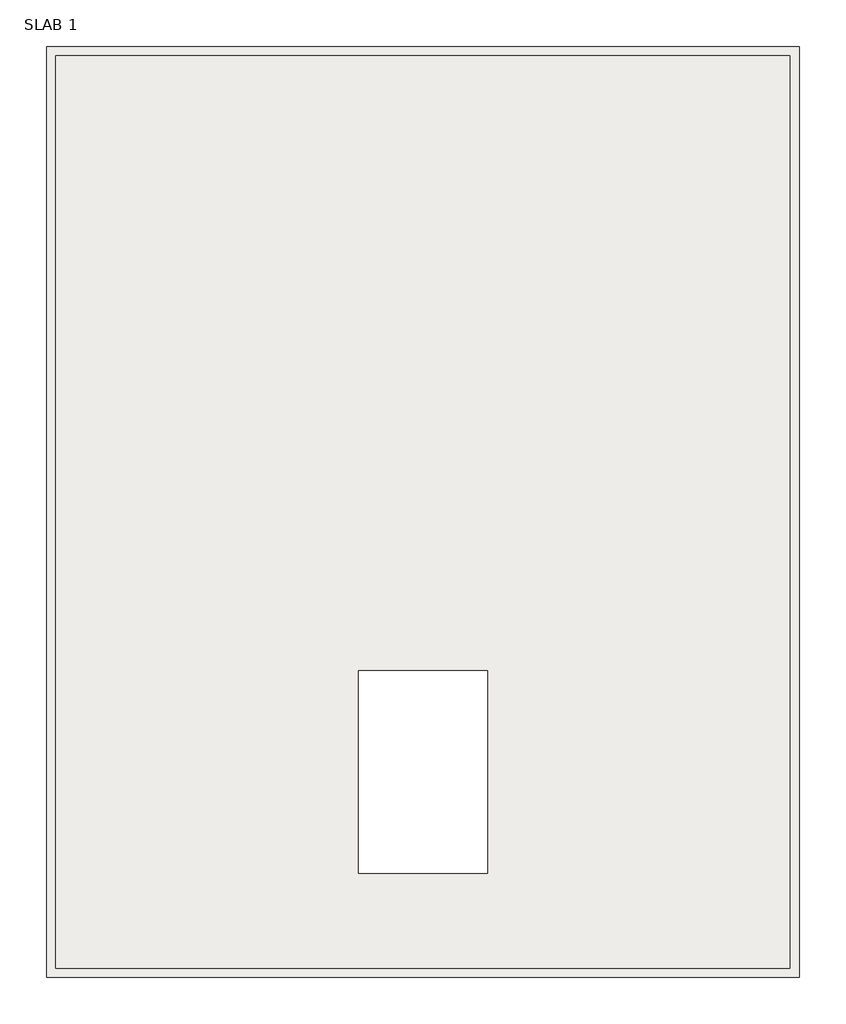
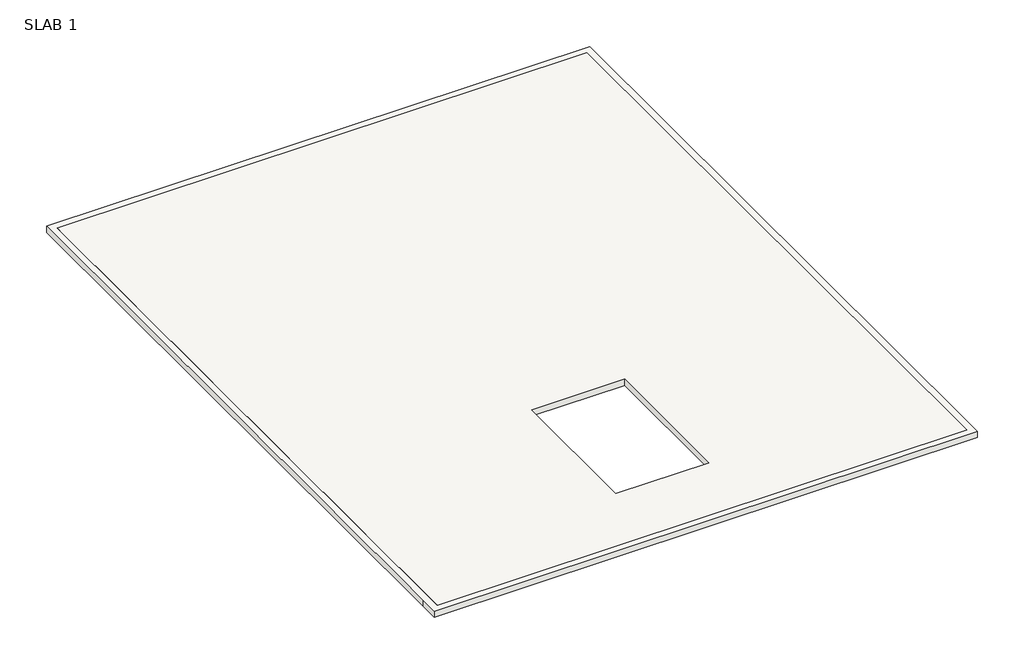
# One storey: 2 roofs.
"""IFC4 building model written with IfcOpenShell, lengths in millimetres."""

from ifc_helpers import new_model, si_unit, frame, origin, place, context, project, spatial, polyline, outline, extrude, element, save

model = new_model("IFC4")

# Units and contexts
model_context = context("Model", 3, world=origin())
ifc_project = project(units=[si_unit("LENGTHUNIT", "METRE", prefix="MILLI")], contexts=[model_context])

# Site, building, storey
site = spatial("IfcSite", under=ifc_project)
building = spatial("IfcBuilding", under=site)
storey = spatial("IfcBuildingStorey", under=building, Name="SLAB 1", Elevation=3048.0)

# Roofs
placement = place(None, origin())
element("IfcRoof", 1, ObjectType="slab 1 6\"", at=placement, inside=storey, context=model_context, shape_type="SweptSolid", body=[
    extrude(outline(polyline([(-15623.8646954, 8580.7272103), (-3455.6771954, 8580.7272103), (-3455.6771954, -6532.2727897), (-15623.8646954, -6532.2727897), (-15623.8646954, 8580.7272103)]), holes=[polyline([(-10605.7771954, -4957.4727897), (-8472.1771954, -4957.4727897), (-8472.1771954, -1604.6727897), (-10605.7771954, -1604.6727897), (-10605.7771954, -4957.4727897)])]), frame((0.0, 0.0, 3048.0), z_axis=(0.0, 0.0, 1.0), x_axis=(1.0, 0.0, 0.0)), (0.0, 0.0, 1.0), 152.4),
])
element("IfcRoof", 2, ObjectType="slab 1 6\"", at=placement, inside=storey, context=model_context, shape_type="SweptSolid", body=[
    extrude(outline(polyline([(-15776.2646954, 8733.1272103), (-3303.2771954, 8733.1272103), (-3303.2771954, -6379.8727897), (-3303.2771954, -6684.6727897), (-15776.2646954, -6684.6727897), (-15776.2646954, -6227.4727897), (-15776.2646954, 8733.1272103)]), holes=[polyline([(-10605.7771954, -4957.4727897), (-8472.1771954, -4957.4727897), (-8472.1771954, -1604.6727897), (-10605.7771954, -1604.6727897), (-10605.7771954, -4957.4727897)])]), frame((0.0, 0.0, 3048.0), z_axis=(0.0, 0.0, 1.0), x_axis=(1.0, 0.0, 0.0)), (0.0, 0.0, 1.0), 152.4),
])

save(model, "model.ifc")

# Revit data of these elements
# Type "slab 1 6\""
#   Assembly Code = "B1020"
#   Layers, outside or top first: 0' - 6" "slab colour" (function 1)
# Element 1 (IfcRoof, "slab 1 6\"")
#   built-in parameter 1001705 = 10.5 (stored number, unit not read)
#   built-in parameter 1001710 = 33615
#   Phase Created = New Construction
#   Materials on its faces: "slab colour", "Porcelain, Linen"
# Element 2 (IfcRoof, "slab 1 6\"")
#   built-in parameter 1001705 = 10.5 (stored number, unit not read)
#   built-in parameter 1001710 = 33615
#   Phase Created = New Construction
#   Materials on its faces: "Porcelain, Linen", "slab colour", "Laminate, Linen, Matte", "Porcelain, Ivory"
# Materials
#   "slab colour": class "Generic", colour RGB 120 120 120, transparency 0, Cost = 0
#   "Porcelain, Linen": class "Ceramic", colour RGB 249 239 230, transparency 0, Description = "Porcelain, linen", Cost = 0
#   "Laminate, Linen, Matte": class "Plastic", colour RGB 249 239 230, transparency 0, Description = "Plastic Laminate - Linen, Matte", Cost = 0
#   "Porcelain, Ivory": class "Ceramic", colour RGB 247 247 239, transparency 0, Description = "Porcelain, ivory", Cost = 0
